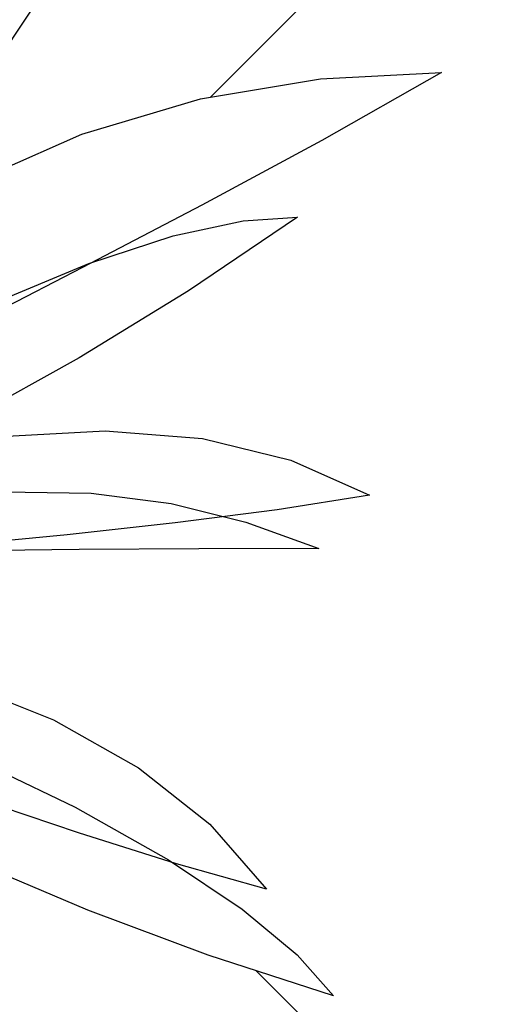
# Model space of a CAD drawing. Units: inches. Extents: x 3590 to 5167, y 65 to 1917.
# Tile 52 of 100: x 4960.64 to 4967.82, y 1515.58 to 1530.53. Entities that reach past the tile are written whole.
import ezdxf

# ---------------------------------------------------------------- set-up
doc = ezdxf.new("R2010")
doc.units = ezdxf.units.IN
doc.layers.add('A-FLOR-PATT', color=8, linetype='Continuous', lineweight=13)
doc.layers.add('L-PLNT', color=94, linetype='Continuous', lineweight=18)
doc.layers.add('DIENHOA', color=3, linetype='Continuous')

# ---------------------------------------------------------------- blocks, each defined once
blk = doc.blocks.new('Cay03_mb')
at = {"layer": 'DIENHOA'}
for p, q in [((510.97, 309.61), (585.91, 313.53)), ((585.91, 313.53), (511.78, 271.41)), ((436.81, 297.21), (510.97, 309.61)), ((363.38, 275.41), (436.81, 297.21)), ((290.63, 243.24), (363.38, 275.41)), ((511.78, 271.41), (437.63, 231.46)), ((437.63, 231.46), (363.69, 192.89)), ((363.69, 192.89), (290.19, 154.87)), ((314.63, 54.14), (369.18, 53.28)), ((369.18, 53.28), (418.6, 46.82)), ((418.6, 46.82), (464.87, 35.24)), ((464.87, 35.24), (510, 19)), ((361.61, 18.5), (289.03, 17.44)), ((435.8, 18.92), (361.61, 18.5)), ((510, 19), (435.8, 18.92)), ((289.55, -107.64), (359.29, -141.1)), ((359.29, -141.1), (416.89, -173.51)), ((367.1, -204.83), (296, -174.69)), ((416.89, -173.51), (462.55, -204.2)), ((441.55, -232.67), (367.1, -204.83)), ((462.55, -204.2), (496.5, -232.48)), ((518.93, -257.68), (441.55, -232.67)), ((496.5, -232.48), (518.93, -257.68))]:
    blk.add_line(p, q, dxfattribs=at)
for points in [[(384.28, 437.45), (342.25, 367.83), (298.14, 301.71), (252.56, 239.37), (206.11, 181.11), (159.39, 127.21), (113.01, 77.96), (67.57, 33.64), (23.69, -5.44)], [(496.74, 224.01), (429.38, 178.44), (361.6, 136.93), (294.07, 99.46), (227.46, 66.07), (162.44, 36.74), (99.68, 11.49), (39.84, -9.67), (-16.39, -26.73)], [(-16.39, -26.73), (75.38, 37.88), (160.06, 91.82), (237.27, 135.67), (306.57, 170.01), (367.58, 195.44), (419.88, 212.52), (463.07, 221.85), (496.74, 224.01)], [(23.69, -5.44), (99.27, 29.67), (173.22, 57.09), (244.79, 76.69), (313.26, 88.31), (377.88, 91.81), (437.93, 87.02), (492.67, 73.8), (541.37, 52)], [(541.37, 52), (484.11, 42.89), (421.18, 34.83), (354.36, 27.58), (285.41, 20.89), (216.1, 14.49), (148.2, 8.14), (83.47, 1.58), (23.69, -5.44)], [(-16.39, -26.73), (66.95, -26.58), (145.58, -32.71), (218.77, -44.94), (285.79, -63.12), (345.92, -87.06), (398.42, -116.6), (442.57, -151.57), (477.63, -191.79)], [(477.63, -191.79), (421.82, -176.03), (361.32, -156.94), (297.62, -135.49), (232.22, -112.64), (166.63, -89.37), (102.33, -66.65), (40.82, -45.45), (-16.39, -26.73)]]:
    blk.add_lwpolyline(points, dxfattribs=at)

msp = doc.modelspace()

# ---------------------------------------------------------------- hatches: boundary and pattern name
at = {"layer": 'A-FLOR-PATT', "transparency": 33554687}
h = msp.add_hatch(dxfattribs=at)
h.set_pattern_fill('AR-HBONE', color=256, scale=0.2)
h.set_pattern_definition([(45, (-588.972, 0), (0, 28.73682), [60.96, -20.32]), (135, (-574.604, 14.368), (3e-15, 28.73682), [60.96, -20.32])])
h.paths.add_polyline_path([(5071.274, 1796.999), (4933.274, 1796.999), (4933.274, 1753.999), (4962.774, 1753.999, -0.414214), (4928.774, 1719.999), (4933.274, 1718.999), (4933.274, 1334.999), (5071.274, 1334.999)])
h.paths.add_polyline_path([(4951.78, 1521.077), (4951.715, 1521.04), (4951.563, 1520.895)], flags=16)
h.paths.add_polyline_path([(4952.267, 1521.376), (4952.198, 1521.371), (4952.198, 1521.356)], flags=0)
h.paths.add_polyline_path([(4967.051, 1529.728), (4965.231, 1528.694), (4963.411, 1527.714), (4961.756, 1526.851), (4963.589, 1527.449), (4964.036, 1527.478), (4962.975, 1527.249), (4961.76, 1526.852), (4959.792, 1525.834), (4958.005, 1524.895), (4956.24, 1523.93), (4954.504, 1522.919), (4954.129, 1522.682), (4953.361, 1521.997), (4953.366, 1521.998), (4953.605, 1522.064), (4955.106, 1522.761), (4956.921, 1523.434), (4958.678, 1523.915), (4960.358, 1524.2), (4961.945, 1524.286), (4964.171, 1524.108), (4965.958, 1523.309), (4963.863, 1522.976), (4965.187, 1522.499), (4963.366, 1522.497), (4961.545, 1522.487), (4959.764, 1522.461), (4958.304, 1522.419), (4957.974, 1522.388), (4956.307, 1522.232), (4954.718, 1522.071), (4953.251, 1521.899), (4953.525, 1521.623), (4954.331, 1521.379), (4956.243, 1521.23), (4958.039, 1520.93), (4959.684, 1520.483), (4961.16, 1519.896), (4963.107, 1518.8), (4964.393, 1517.325), (4962.973, 1517.726), (4964.558, 1516.661), (4965.407, 1515.708), (4963.507, 1516.322), (4961.68, 1517.005), (4959.935, 1517.745), (4958.282, 1518.528), (4956.732, 1519.343), (4955.295, 1520.175), (4954.672, 1520.572), (4954.513, 1520.627), (4955.658, 1519.318), (4956.703, 1517.982), (4957.644, 1516.647), (4958.485, 1515.334), (4959.55, 1513.524), (4960.438, 1511.769), (4958.841, 1513.62), (4957.452, 1515.325), (4955.819, 1517.459), (4956.665, 1515.448), (4957.111, 1513.923), (4957.447, 1511.714), (4957.076, 1509.793), (4956.538, 1511.11), (4955.992, 1512.569), (4955.444, 1514.125), (4954.898, 1515.735), (4954.357, 1517.356), (4953.824, 1518.943), (4953.305, 1520.452), (4953.065, 1521.116), (4952.971, 1521.146), (4952.949, 1521.086), (4952.73, 1520.199), (4953.37, 1518.024), (4953.757, 1516.373), (4954.051, 1514.765), (4954.264, 1513.221), (4954.471, 1511.131), (4954.497, 1510.402), (4954.409, 1511.76), (4954.264, 1513.221), (4954.051, 1514.765), (4953.757, 1516.373), (4953.37, 1518.024), (4952.877, 1519.698), (4952.716, 1520.141), (4952.533, 1519.059), (4952.374, 1517.789), (4952.219, 1516.312), (4952.046, 1514.6), (4951.833, 1512.626), (4951.557, 1510.363), (4951.203, 1512.168), (4950.852, 1514.339), (4950.985, 1516.376), (4951.66, 1518.286), (4952.593, 1520.481), (4952.357, 1521.13), (4951.855, 1520.328), (4950.839, 1518.908), (4949.777, 1517.587), (4948.916, 1516.617), (4948.111, 1515.256), (4947.089, 1513.554), (4945.889, 1511.615), (4946.326, 1513.402), (4946.562, 1514.249), (4945.528, 1513.327), (4944.581, 1512.531), (4946.018, 1514.508), (4947.204, 1516.048), (4947.893, 1517.313), (4949.307, 1518.764), (4950.414, 1519.767), (4950.451, 1519.806), (4952.267, 1521.376), (4951.645, 1521.493), (4950.404, 1521.18), (4948.044, 1520.359), (4946.119, 1519.452), (4944.572, 1518.475), (4943.35, 1517.443), (4941.997, 1515.92), (4941.661, 1515.275), (4942.813, 1516.99), (4944.572, 1518.475), (4946.119, 1519.452), (4948.044, 1520.359), (4950.404, 1521.18), (4951.645, 1521.493), (4949.647, 1521.868), (4948.6, 1521.756), (4947.126, 1521.57), (4945.42, 1521.348), (4943.45, 1521.105), (4941.183, 1520.856), (4942.86, 1521.613), (4943.873, 1522.03), (4942.952, 1521.909), (4941.41, 1521.485), (4939.543, 1520.67), (4938.968, 1520.226), (4940.733, 1521.299), (4942.952, 1521.909), (4943.702, 1522.008), (4945.894, 1522.7), (4947.565, 1522.714), (4948.921, 1522.566), (4951.131, 1522.183), (4950.971, 1522.297), (4948.129, 1523.006), (4946.035, 1523.707), (4944.232, 1524.521), (4942.707, 1525.461), (4941.444, 1526.537), (4940.43, 1527.761), (4939.649, 1529.143), (4941.421, 1528.122), (4943.147, 1527.132), (4944.841, 1526.175), (4946.514, 1525.25), (4948.179, 1524.359), (4948.365, 1524.263), (4946.475, 1526.045), (4945.181, 1527.54), (4944.19, 1529.033), (4943.496, 1530.54), (4943.278, 1531.36), (4942.498, 1531.919), (4943.114, 1531.762), (4942.959, 1533.659), (4944.14, 1531.989), (4944.612, 1531.323), (4946.202, 1530.463), (4947.486, 1529.509), (4948.79, 1528.226), (4950.368, 1526.237), (4949.485, 1528.155), (4948.851, 1530.123), (4948.491, 1532.041), (4948.381, 1533.918), (4948.501, 1535.76), (4948.827, 1537.573), (4949.418, 1535.565), (4949.957, 1533.569), (4950.464, 1531.586), (4950.961, 1529.617), (4951.391, 1527.954), (4951.724, 1530.687), (4952.201, 1532.58), (4952.889, 1534.33), (4953.77, 1535.951), (4954.827, 1537.46), (4954.521, 1535.39), (4954.273, 1533.937), (4955.58, 1535.663), (4956.748, 1536.739), (4956.159, 1534.78), (4955.589, 1532.873), (4955.043, 1531.006), (4954.525, 1529.166), (4954.038, 1527.341), (4953.638, 1525.733), (4953.611, 1525.586), (4953.398, 1524.166), (4953.382, 1524.009), (4954.07, 1525.476), (4954.912, 1527.022), (4956.136, 1528.894), (4957.847, 1530.577), (4959.376, 1531.54), (4958.256, 1530.104), (4957.143, 1528.663), (4956.066, 1527.243), (4955.056, 1525.871), (4954.141, 1524.571), (4953.352, 1523.372), (4953.311, 1523.303), (4953.273, 1522.925), (4953.261, 1522.382), (4954.103, 1523.373), (4954.63, 1524.284), (4955.961, 1526.358), (4957.23, 1528.13), (4958.421, 1529.609), (4960.037, 1531.368), (4961.374, 1532.375), (4962.101, 1532.77), (4961.07, 1531.061), (4959.987, 1529.438), (4958.869, 1527.908), (4958.15, 1527.007), (4959.803, 1528.003), (4961.589, 1528.793), (4963.391, 1529.328), (4965.211, 1529.632)], flags=16)
h.paths.add_polyline_path([(4962.944, 1523.182), (4961.107, 1523.422), (4960.392, 1523.362), (4962.35, 1523.331)], flags=0)
h.paths.add_polyline_path([(5049.541, 1584.551), (5049.476, 1584.515), (5049.325, 1584.37)], flags=16)
h.paths.add_polyline_path([(5050.028, 1584.851), (5049.959, 1584.845), (5049.959, 1584.83)], flags=0)
h.paths.add_polyline_path([(5042.333, 1581.949), (5043.88, 1582.926), (5045.806, 1583.833), (5048.165, 1584.654), (5049.406, 1584.967), (5047.408, 1585.342), (5046.361, 1585.231), (5044.888, 1585.044), (5043.181, 1584.822), (5041.211, 1584.579), (5038.944, 1584.33), (5040.622, 1585.087), (5041.634, 1585.504), (5040.713, 1585.383), (5039.171, 1584.959), (5037.304, 1584.144), (5036.729, 1583.7), (5038.494, 1584.773), (5040.713, 1585.383), (5041.463, 1585.482), (5043.655, 1586.174), (5045.326, 1586.188), (5046.682, 1586.04), (5048.893, 1585.657), (5048.732, 1585.771), (5045.891, 1586.48), (5043.796, 1587.181), (5041.994, 1587.996), (5040.468, 1588.935), (5039.205, 1590.011), (5038.191, 1591.235), (5037.41, 1592.617), (5039.182, 1591.596), (5040.909, 1590.607), (5042.602, 1589.649), (5044.275, 1588.724), (5045.94, 1587.833), (5046.126, 1587.738), (5044.237, 1589.519), (5042.942, 1591.015), (5041.952, 1592.508), (5041.257, 1594.014), (5041.039, 1594.834), (5040.26, 1595.393), (5040.875, 1595.237), (5040.721, 1597.133), (5041.901, 1595.463), (5042.373, 1594.798), (5043.963, 1593.938), (5045.247, 1592.983), (5046.552, 1591.701), (5048.129, 1589.712), (5047.247, 1591.63), (5046.613, 1593.597), (5046.252, 1595.515), (5046.142, 1597.392), (5046.262, 1599.234), (5046.588, 1601.047), (5047.179, 1599.039), (5047.718, 1597.043), (5048.225, 1595.06), (5048.722, 1593.091), (5049.152, 1591.429), (5049.485, 1594.161), (5049.962, 1596.054), (5050.65, 1597.804), (5051.532, 1599.425), (5052.589, 1600.934), (5052.283, 1598.864), (5052.034, 1597.411), (5053.341, 1599.137), (5054.509, 1600.213), (5053.92, 1598.254), (5053.35, 1596.348), (5052.805, 1594.48), (5052.286, 1592.64), (5051.799, 1590.815), (5051.4, 1589.207), (5051.373, 1589.06), (5051.159, 1587.64), (5051.143, 1587.483), (5051.831, 1588.95), (5052.673, 1590.496), (5053.898, 1592.368), (5055.608, 1594.051), (5057.137, 1595.014), (5056.017, 1593.578), (5054.904, 1592.137), (5053.828, 1590.717), (5052.817, 1589.345), (5051.902, 1588.046), (5051.113, 1586.846), (5051.072, 1586.777), (5051.034, 1586.399), (5051.022, 1585.856), (5051.864, 1586.847), (5052.391, 1587.758), (5053.723, 1589.832), (5054.991, 1591.604), (5056.182, 1593.083), (5057.798, 1594.842), (5059.135, 1595.849), (5059.863, 1596.244), (5058.831, 1594.535), (5057.749, 1592.912), (5056.63, 1591.382), (5055.912, 1590.482), (5057.564, 1591.477), (5059.35, 1592.267), (5061.152, 1592.802), (5062.972, 1593.106), (5064.812, 1593.203), (5062.992, 1592.169), (5061.172, 1591.188), (5059.518, 1590.325), (5061.35, 1590.924), (5061.797, 1590.952), (5060.737, 1590.723), (5059.521, 1590.326), (5057.553, 1589.308), (5055.766, 1588.369), (5054.002, 1587.404), (5052.265, 1586.393), (5051.891, 1586.156), (5051.122, 1585.471), (5051.127, 1585.472), (5051.366, 1585.538), (5052.867, 1586.235), (5054.682, 1586.908), (5056.439, 1587.389), (5058.12, 1587.675), (5059.706, 1587.76), (5061.933, 1587.583), (5063.719, 1586.783), (5061.624, 1586.45), (5062.949, 1585.973), (5061.127, 1585.971), (5059.307, 1585.961), (5057.525, 1585.935), (5056.065, 1585.893), (5055.735, 1585.862), (5054.068, 1585.707), (5052.479, 1585.546), (5051.012, 1585.373), (5051.286, 1585.097), (5052.092, 1584.853), (5054.004, 1584.704), (5055.8, 1584.404), (5057.446, 1583.958), (5058.921, 1583.37), (5060.868, 1582.274), (5062.154, 1580.799), (5060.734, 1581.2), (5062.32, 1580.135), (5063.168, 1579.182), (5061.269, 1579.796), (5059.441, 1580.479), (5057.696, 1581.219), (5056.043, 1582.003), (5054.493, 1582.817), (5053.057, 1583.649), (5052.433, 1584.047), (5052.274, 1584.101), (5053.42, 1582.793), (5054.464, 1581.457), (5055.405, 1580.121), (5056.247, 1578.809), (5057.311, 1576.998), (5058.199, 1575.244), (5056.602, 1577.094), (5055.213, 1578.799), (5053.58, 1580.933), (5054.427, 1578.922), (5054.872, 1577.397), (5055.208, 1575.189), (5054.838, 1573.267), (5054.299, 1574.584), (5053.754, 1576.043), (5053.206, 1577.599), (5052.659, 1579.209), (5052.118, 1580.83), (5051.585, 1582.417), (5051.066, 1583.927), (5050.826, 1584.59), (5050.733, 1584.62), (5050.711, 1584.561), (5050.491, 1583.673), (5051.131, 1581.498), (5051.518, 1579.847), (5051.813, 1578.24), (5052.026, 1576.695), (5052.233, 1574.605), (5052.258, 1573.876), (5052.17, 1575.234), (5052.026, 1576.695), (5051.813, 1578.24), (5051.518, 1579.847), (5051.131, 1581.498), (5050.638, 1583.172), (5050.477, 1583.615), (5050.294, 1582.533), (5050.136, 1581.263), (5049.981, 1579.786), (5049.807, 1578.074), (5049.594, 1576.1), (5049.318, 1573.837), (5048.965, 1575.642), (5048.613, 1577.813), (5048.747, 1579.85), (5049.421, 1581.76), (5050.354, 1583.955), (5050.118, 1584.604), (5049.616, 1583.802), (5048.6, 1582.382), (5047.538, 1581.061), (5046.677, 1580.091), (5045.872, 1578.73), (5044.85, 1577.028), (5043.651, 1575.089), (5044.087, 1576.877), (5044.324, 1577.723), (5043.289, 1576.801), (5042.342, 1576.005), (5043.779, 1577.982), (5044.966, 1579.522), (5045.655, 1580.787), (5047.068, 1582.239), (5048.175, 1583.241), (5048.213, 1583.28), (5050.028, 1584.851), (5049.406, 1584.967), (5048.165, 1584.654), (5045.806, 1583.833), (5043.88, 1582.926), (5042.333, 1581.949), (5041.111, 1580.917), (5039.758, 1579.394), (5039.423, 1578.749), (5040.575, 1580.464)], flags=16)
h.paths.add_polyline_path([(4954.799, 1533.12), (4954.262, 1532.079), (4953.831, 1530.935), (4953.505, 1529.636), (4953.283, 1528.133), (4953.167, 1526.376), (4953.156, 1524.315), (4953.277, 1521.236), (4952.802, 1521.842), (4951.557, 1521.998), (4950.976, 1521.961), (4952.661, 1521.941), (4952.802, 1521.842), (4953.152, 1523.593), (4953.167, 1526.376), (4953.283, 1528.133), (4953.609, 1530.346), (4954.456, 1532.592)], flags=0)
h.paths.add_polyline_path([(5050.563, 1585.316), (5049.318, 1585.472), (5048.737, 1585.435), (5050.422, 1585.415), (5050.563, 1585.316), (5050.914, 1587.067), (5050.928, 1589.851), (5051.045, 1591.607), (5051.371, 1593.82), (5052.217, 1596.066), (5052.56, 1596.594), (5052.024, 1595.554), (5051.592, 1594.409), (5051.266, 1593.11), (5051.045, 1591.607), (5050.928, 1589.851), (5050.918, 1587.789), (5051.038, 1584.71)], flags=0)
h.paths.add_polyline_path([(5058.153, 1586.836), (5060.111, 1586.805), (5060.705, 1586.656), (5058.868, 1586.896)], flags=0)
h.paths.add_polyline_path([(5049.541, 1430.936), (5049.476, 1430.9), (5049.325, 1430.755)], flags=16)
h.paths.add_polyline_path([(5050.028, 1431.236), (5049.959, 1431.231), (5049.959, 1431.215)], flags=0)
h.paths.add_polyline_path([(5046.588, 1447.432), (5047.179, 1445.425), (5047.718, 1443.429), (5048.225, 1441.446), (5048.722, 1439.476), (5049.152, 1437.814), (5049.485, 1440.546), (5049.962, 1442.439), (5050.65, 1444.189), (5051.532, 1445.811), (5052.589, 1447.319), (5052.283, 1445.249), (5052.034, 1443.796), (5053.341, 1445.522), (5054.509, 1446.598), (5053.92, 1444.64), (5053.35, 1442.733), (5052.805, 1440.865), (5052.286, 1439.025), (5051.799, 1437.201), (5051.4, 1435.592), (5051.373, 1435.445), (5051.159, 1434.025), (5051.143, 1433.868), (5051.831, 1435.335), (5052.673, 1436.881), (5053.898, 1438.753), (5055.608, 1440.436), (5057.137, 1441.4), (5056.017, 1439.963), (5054.904, 1438.522), (5053.828, 1437.102), (5052.817, 1435.73), (5051.902, 1434.431), (5051.113, 1433.231), (5051.072, 1433.162), (5051.034, 1432.784), (5051.022, 1432.242), (5051.864, 1433.232), (5052.391, 1434.143), (5053.723, 1436.217), (5054.991, 1437.989), (5056.182, 1439.468), (5057.798, 1441.227), (5059.135, 1442.235), (5059.863, 1442.629), (5058.831, 1440.921), (5057.749, 1439.298), (5056.63, 1437.767), (5055.912, 1436.867), (5057.564, 1437.863), (5059.35, 1438.652), (5061.152, 1439.187), (5062.972, 1439.491), (5064.812, 1439.588), (5062.992, 1438.554), (5061.172, 1437.573), (5059.518, 1436.71), (5061.35, 1437.309), (5061.797, 1437.337), (5060.737, 1437.108), (5059.521, 1436.711), (5057.553, 1435.693), (5055.766, 1434.754), (5054.002, 1433.789), (5052.265, 1432.778), (5051.891, 1432.541), (5051.122, 1431.856), (5051.127, 1431.857), (5051.366, 1431.923), (5052.867, 1432.62), (5054.682, 1433.293), (5056.439, 1433.775), (5058.12, 1434.06), (5059.706, 1434.145), (5061.933, 1433.968), (5063.719, 1433.168), (5061.624, 1432.835), (5062.949, 1432.358), (5061.127, 1432.357), (5059.307, 1432.346), (5057.525, 1432.32), (5056.065, 1432.278), (5055.735, 1432.248), (5054.068, 1432.092), (5052.479, 1431.931), (5051.012, 1431.759), (5051.286, 1431.482), (5052.092, 1431.238), (5054.004, 1431.089), (5055.8, 1430.789), (5057.446, 1430.343), (5058.921, 1429.755), (5060.868, 1428.66), (5062.154, 1427.185), (5060.734, 1427.585), (5062.32, 1426.52), (5063.168, 1425.567), (5061.269, 1426.181), (5059.441, 1426.865), (5057.696, 1427.604), (5056.043, 1428.388), (5054.493, 1429.202), (5053.057, 1430.034), (5052.433, 1430.432), (5052.274, 1430.487), (5053.42, 1429.178), (5054.464, 1427.842), (5055.405, 1426.506), (5056.247, 1425.194), (5057.311, 1423.383), (5058.199, 1421.629), (5056.602, 1423.479), (5055.213, 1425.184), (5053.58, 1427.318), (5054.427, 1425.307), (5054.872, 1423.782), (5055.208, 1421.574), (5054.838, 1419.652), (5054.299, 1420.97), (5053.754, 1422.428), (5053.206, 1423.984), (5052.659, 1425.595), (5052.118, 1427.215), (5051.585, 1428.802), (5051.066, 1430.312), (5050.826, 1430.975), (5050.733, 1431.005), (5050.711, 1430.946), (5050.491, 1430.058), (5051.131, 1427.883), (5051.518, 1426.232), (5051.813, 1424.625), (5052.026, 1423.081), (5052.233, 1420.991), (5052.258, 1420.261), (5052.17, 1421.619), (5052.026, 1423.081), (5051.813, 1424.625), (5051.518, 1426.232), (5051.131, 1427.883), (5050.638, 1429.558), (5050.477, 1430.001), (5050.294, 1428.918), (5050.136, 1427.648), (5049.981, 1426.171), (5049.807, 1424.459), (5049.594, 1422.485), (5049.318, 1420.222), (5048.965, 1422.028), (5048.613, 1424.199), (5048.747, 1426.235), (5049.421, 1428.146), (5050.354, 1430.34), (5050.118, 1430.989), (5049.616, 1430.187), (5048.6, 1428.768), (5047.538, 1427.446), (5046.677, 1426.477), (5045.872, 1425.116), (5044.85, 1423.413), (5043.651, 1421.474), (5044.087, 1423.262), (5044.324, 1424.109), (5043.289, 1423.186), (5042.342, 1422.391), (5043.779, 1424.368), (5044.966, 1425.907), (5045.655, 1427.173), (5047.068, 1428.624), (5048.175, 1429.627), (5048.213, 1429.666), (5050.028, 1431.236), (5049.406, 1431.353), (5048.165, 1431.039), (5045.806, 1430.218), (5043.88, 1429.311), (5042.333, 1428.334), (5041.111, 1427.302), (5039.758, 1425.779), (5039.423, 1425.134), (5040.575, 1426.849), (5042.333, 1428.334), (5043.88, 1429.311), (5045.806, 1430.218), (5048.165, 1431.039), (5049.406, 1431.353), (5047.408, 1431.727), (5046.361, 1431.616), (5044.888, 1431.429), (5043.181, 1431.207), (5041.211, 1430.964), (5038.944, 1430.715), (5040.622, 1431.472), (5041.634, 1431.89), (5040.713, 1431.769), (5039.171, 1431.345), (5037.304, 1430.53), (5036.729, 1430.085), (5038.494, 1431.158), (5040.713, 1431.769), (5041.463, 1431.867), (5043.655, 1432.559), (5045.326, 1432.573), (5046.682, 1432.425), (5048.893, 1432.042), (5048.732, 1432.156), (5045.891, 1432.865), (5043.796, 1433.566), (5041.994, 1434.381), (5040.468, 1435.321), (5039.205, 1436.396), (5038.191, 1437.62), (5037.41, 1439.002), (5039.182, 1437.982), (5040.909, 1436.992), (5042.602, 1436.034), (5044.275, 1435.109), (5045.94, 1434.218), (5046.126, 1434.123), (5044.237, 1435.904), (5042.942, 1437.4), (5041.952, 1438.893), (5041.257, 1440.399), (5041.039, 1441.219), (5040.26, 1441.778), (5040.875, 1441.622), (5040.721, 1443.518), (5041.901, 1441.848), (5042.373, 1441.183), (5043.963, 1440.323), (5045.247, 1439.369), (5046.552, 1438.086), (5048.129, 1436.097), (5047.247, 1438.015), (5046.613, 1439.982), (5046.252, 1441.901), (5046.142, 1443.778), (5046.262, 1445.619)], flags=16)
h.paths.add_polyline_path([(5052.382, 1444.255), (5051.623, 1442.78), (5052.024, 1441.939), (5052.56, 1442.98)], flags=0)
h.paths.add_polyline_path([(5050.563, 1431.701), (5049.318, 1431.857), (5048.737, 1431.821), (5050.422, 1431.8)], flags=0)
h.paths.add_polyline_path([(5058.153, 1433.221), (5060.111, 1433.19), (5060.705, 1433.041), (5058.868, 1433.281)], flags=0)
h.paths.add_polyline_path([(5049.541, 1352.285), (5049.476, 1352.249), (5049.325, 1352.104)], flags=16)
h.paths.add_polyline_path([(5050.028, 1352.585), (5049.959, 1352.58), (5049.959, 1352.564)], flags=0)
h.paths.add_polyline_path([(5046.588, 1368.781), (5047.179, 1366.774), (5047.718, 1364.778), (5048.225, 1362.795), (5048.722, 1360.825), (5049.152, 1359.163), (5049.485, 1361.896), (5049.962, 1363.789), (5050.65, 1365.538), (5051.532, 1367.16), (5052.589, 1368.669), (5052.283, 1366.598), (5052.034, 1365.145), (5053.341, 1366.871), (5054.509, 1367.947), (5053.92, 1365.989), (5053.35, 1364.082), (5052.805, 1362.214), (5052.286, 1360.374), (5051.799, 1358.55), (5051.4, 1356.942), (5051.373, 1356.794), (5051.159, 1355.374), (5051.143, 1355.218), (5051.831, 1356.684), (5052.673, 1358.23), (5053.898, 1360.102), (5055.608, 1361.786), (5057.137, 1362.749), (5056.017, 1361.313), (5054.904, 1359.872), (5053.828, 1358.452), (5052.817, 1357.079), (5051.902, 1355.78), (5051.113, 1354.581), (5051.072, 1354.512), (5051.034, 1354.133), (5051.022, 1353.591), (5051.864, 1354.581), (5052.391, 1355.492), (5053.723, 1357.566), (5054.991, 1359.338), (5056.182, 1360.817), (5057.798, 1362.577), (5059.135, 1363.584), (5059.863, 1363.979), (5058.831, 1362.27), (5057.749, 1360.647), (5056.63, 1359.117), (5055.912, 1358.216), (5057.564, 1359.212), (5059.35, 1360.001), (5061.152, 1360.536), (5062.972, 1360.841), (5064.812, 1360.937), (5062.992, 1359.903), (5061.172, 1358.923), (5059.518, 1358.059), (5061.35, 1358.658), (5061.797, 1358.687), (5060.737, 1358.458), (5059.521, 1358.061), (5057.553, 1357.043), (5055.766, 1356.103), (5054.002, 1355.138), (5052.265, 1354.127), (5051.891, 1353.89), (5051.122, 1353.206), (5051.127, 1353.206), (5051.366, 1353.272), (5052.867, 1353.969), (5054.682, 1354.643), (5056.439, 1355.124), (5058.12, 1355.409), (5059.706, 1355.495), (5061.933, 1355.317), (5063.719, 1354.518), (5061.624, 1354.184), (5062.949, 1353.708), (5061.127, 1353.706), (5059.307, 1353.695), (5057.525, 1353.669), (5056.065, 1353.627), (5055.735, 1353.597), (5054.068, 1353.441), (5052.479, 1353.28), (5051.012, 1353.108), (5051.286, 1352.831), (5052.092, 1352.587), (5054.004, 1352.439), (5055.8, 1352.138), (5057.446, 1351.692), (5058.921, 1351.104), (5060.868, 1350.009), (5062.154, 1348.534), (5060.734, 1348.935), (5062.32, 1347.869), (5063.168, 1346.916), (5061.269, 1347.53), (5059.441, 1348.214), (5057.696, 1348.954), (5056.043, 1349.737), (5054.493, 1350.551), (5053.057, 1351.383), (5052.433, 1351.781), (5052.274, 1351.836), (5053.42, 1350.527), (5054.464, 1349.191), (5055.405, 1347.855), (5056.247, 1346.543), (5057.311, 1344.733), (5058.199, 1342.978), (5056.602, 1344.828), (5055.213, 1346.534), (5053.58, 1348.667), (5054.427, 1346.656), (5054.872, 1345.132), (5055.208, 1342.923), (5054.838, 1341.002), (5054.299, 1342.319), (5053.754, 1343.778), (5053.206, 1345.334), (5052.659, 1346.944), (5052.118, 1348.564), (5051.585, 1350.151), (5051.066, 1351.661), (5050.826, 1352.324), (5050.733, 1352.355), (5050.711, 1352.295), (5050.491, 1351.408), (5051.131, 1349.232), (5051.518, 1347.581), (5051.813, 1345.974), (5052.026, 1344.43), (5052.233, 1342.34), (5052.258, 1341.61), (5052.17, 1342.969), (5052.026, 1344.43), (5051.813, 1345.974), (5051.518, 1347.581), (5051.131, 1349.232), (5050.638, 1350.907), (5050.477, 1351.35), (5050.294, 1350.267), (5050.136, 1348.997), (5049.981, 1347.52), (5049.807, 1345.809), (5049.594, 1343.835), (5049.318, 1341.571), (5048.965, 1343.377), (5048.613, 1345.548), (5048.747, 1347.585), (5049.421, 1349.495), (5050.354, 1351.689), (5050.118, 1352.339), (5049.616, 1351.536), (5048.6, 1350.117), (5047.538, 1348.795), (5046.677, 1347.826), (5045.872, 1346.465), (5044.85, 1344.763), (5043.651, 1342.824), (5044.087, 1344.611), (5044.324, 1345.458), (5043.289, 1344.535), (5042.342, 1343.74), (5043.779, 1345.717), (5044.966, 1347.256), (5045.655, 1348.522), (5047.068, 1349.973), (5048.175, 1350.976), (5048.213, 1351.015), (5050.028, 1352.585), (5049.406, 1352.702), (5048.165, 1352.388), (5045.806, 1351.567), (5043.88, 1350.661), (5042.333, 1349.683), (5041.111, 1348.651), (5039.758, 1347.128), (5039.423, 1346.483), (5040.575, 1348.198), (5042.333, 1349.683), (5043.88, 1350.661), (5045.806, 1351.567), (5048.165, 1352.388), (5049.406, 1352.702), (5047.408, 1353.076), (5046.361, 1352.965), (5044.888, 1352.779), (5043.181, 1352.556), (5041.211, 1352.313), (5038.944, 1352.065), (5040.622, 1352.821), (5041.634, 1353.239), (5040.713, 1353.118), (5039.171, 1352.694), (5037.304, 1351.879), (5036.729, 1351.434), (5038.494, 1352.508), (5040.713, 1353.118), (5041.463, 1353.216), (5043.655, 1353.909), (5045.326, 1353.923), (5046.682, 1353.774), (5048.893, 1353.391), (5048.732, 1353.506), (5045.891, 1354.214), (5043.796, 1354.915), (5041.994, 1355.73), (5040.468, 1356.67), (5039.205, 1357.746), (5038.191, 1358.969), (5037.41, 1360.352), (5039.182, 1359.331), (5040.909, 1358.341), (5042.602, 1357.383), (5044.275, 1356.458), (5045.94, 1355.567), (5046.126, 1355.472), (5044.237, 1357.253), (5042.942, 1358.749), (5041.952, 1360.242), (5041.257, 1361.748), (5041.039, 1362.568), (5040.26, 1363.128), (5040.875, 1362.971), (5040.721, 1364.867), (5041.901, 1363.197), (5042.373, 1362.532), (5043.963, 1361.672), (5045.247, 1360.718), (5046.552, 1359.435), (5048.129, 1357.446), (5047.247, 1359.364), (5046.613, 1361.331), (5046.252, 1363.25), (5046.142, 1365.127), (5046.262, 1366.969)], flags=16)
h.paths.add_polyline_path([(5052.382, 1365.604), (5051.623, 1364.129), (5052.024, 1363.288), (5052.56, 1364.329)], flags=0)
h.paths.add_polyline_path([(4951.78, 1698.041), (4951.715, 1698.005), (4951.563, 1697.859)], flags=16)
h.paths.add_polyline_path([(4952.267, 1698.341), (4952.198, 1698.335), (4952.198, 1698.32)], flags=0)
h.paths.add_polyline_path([(4957.076, 1686.757), (4956.538, 1688.074), (4955.992, 1689.533), (4955.444, 1691.089), (4954.898, 1692.699), (4954.357, 1694.32), (4953.824, 1695.907), (4953.305, 1697.417), (4953.065, 1698.08), (4952.971, 1698.11), (4952.949, 1698.051), (4952.73, 1697.163), (4953.37, 1694.988), (4953.757, 1693.337), (4954.051, 1691.729), (4954.264, 1690.185), (4954.471, 1688.095), (4954.497, 1687.366), (4954.409, 1688.724), (4954.264, 1690.185), (4954.051, 1691.729), (4953.757, 1693.337), (4953.37, 1694.988), (4952.877, 1696.662), (4952.716, 1697.105), (4952.533, 1696.023), (4952.374, 1694.753), (4952.219, 1693.276), (4952.046, 1691.564), (4951.833, 1689.59), (4951.557, 1687.327), (4951.203, 1689.132), (4950.852, 1691.303), (4950.985, 1693.34), (4951.66, 1695.25), (4952.593, 1697.445), (4952.357, 1698.094), (4951.855, 1697.292), (4950.839, 1695.872), (4949.777, 1694.551), (4948.916, 1693.581), (4948.111, 1692.22), (4947.089, 1690.518), (4945.889, 1688.579), (4946.326, 1690.366), (4946.562, 1691.213), (4945.528, 1690.291), (4944.581, 1689.495), (4946.018, 1691.472), (4947.204, 1693.012), (4947.893, 1694.277), (4949.307, 1695.729), (4950.414, 1696.731), (4950.451, 1696.77), (4952.267, 1698.341), (4951.645, 1698.457), (4950.404, 1698.144), (4948.044, 1697.323), (4946.119, 1696.416), (4944.572, 1695.439), (4943.35, 1694.407), (4941.997, 1692.884), (4941.661, 1692.239), (4942.813, 1693.954), (4944.572, 1695.439), (4946.119, 1696.416), (4948.044, 1697.323), (4950.404, 1698.144), (4951.645, 1698.457), (4949.647, 1698.832), (4948.6, 1698.72), (4947.126, 1698.534), (4945.42, 1698.312), (4943.45, 1698.069), (4941.183, 1697.82), (4942.86, 1698.577), (4943.873, 1698.994), (4942.952, 1698.873), (4941.41, 1698.449), (4939.543, 1697.634), (4938.968, 1697.19), (4940.733, 1698.263), (4942.952, 1698.873), (4943.702, 1698.972), (4945.894, 1699.664), (4947.565, 1699.678), (4948.921, 1699.53), (4951.131, 1699.147), (4950.971, 1699.261), (4948.129, 1699.97), (4946.035, 1700.671), (4944.232, 1701.486), (4942.707, 1702.425), (4941.444, 1703.501), (4940.43, 1704.725), (4939.649, 1706.107), (4941.421, 1705.086), (4943.147, 1704.097), (4944.841, 1703.139), (4946.514, 1702.214), (4948.179, 1701.323), (4948.365, 1701.227), (4946.475, 1703.009), (4945.181, 1704.505), (4944.19, 1705.997), (4943.496, 1707.504), (4943.278, 1708.324), (4942.498, 1708.883), (4943.114, 1708.727), (4942.959, 1710.623), (4944.14, 1708.953), (4944.612, 1708.287), (4946.202, 1707.428), (4947.486, 1706.473), (4948.79, 1705.191), (4950.368, 1703.202), (4949.485, 1705.12), (4948.851, 1707.087), (4948.491, 1709.005), (4948.381, 1710.882), (4948.501, 1712.724), (4948.827, 1714.537), (4949.418, 1712.529), (4949.957, 1710.533), (4950.464, 1708.55), (4950.961, 1706.581), (4951.391, 1704.919), (4951.724, 1707.651), (4952.201, 1709.544), (4952.889, 1711.294), (4953.77, 1712.915), (4954.827, 1714.424), (4954.521, 1712.354), (4954.273, 1710.901), (4955.58, 1712.627), (4956.748, 1713.703), (4956.159, 1711.744), (4955.589, 1709.837), (4955.043, 1707.97), (4954.525, 1706.13), (4954.038, 1704.305), (4953.638, 1702.697), (4953.611, 1702.55), (4953.398, 1701.13), (4953.382, 1700.973), (4954.07, 1702.44), (4954.912, 1703.986), (4956.136, 1705.858), (4957.847, 1707.541), (4959.376, 1708.504), (4958.256, 1707.068), (4957.143, 1705.627), (4956.066, 1704.207), (4955.056, 1702.835), (4954.141, 1701.536), (4953.352, 1700.336), (4953.311, 1700.267), (4953.273, 1699.889), (4953.261, 1699.346), (4954.103, 1700.337), (4954.63, 1701.248), (4955.961, 1703.322), (4957.23, 1705.094), (4958.421, 1706.573), (4960.037, 1708.332), (4961.374, 1709.339), (4962.101, 1709.734), (4961.07, 1708.025), (4959.987, 1706.402), (4958.869, 1704.872), (4958.15, 1703.972), (4959.803, 1704.967), (4961.589, 1705.757), (4963.391, 1706.292), (4965.211, 1706.596), (4967.051, 1706.692), (4965.231, 1705.659), (4963.411, 1704.678), (4961.756, 1703.815), (4963.589, 1704.413), (4964.036, 1704.442), (4962.975, 1704.213), (4961.76, 1703.816), (4959.792, 1702.798), (4958.005, 1701.859), (4956.24, 1700.894), (4954.504, 1699.883), (4954.129, 1699.646), (4953.361, 1698.961), (4953.366, 1698.962), (4953.605, 1699.028), (4955.106, 1699.725), (4956.921, 1700.398), (4958.678, 1700.879), (4960.358, 1701.164), (4961.945, 1701.25), (4964.171, 1701.073), (4965.958, 1700.273), (4963.863, 1699.94), (4965.187, 1699.463), (4963.366, 1699.461), (4961.545, 1699.451), (4959.764, 1699.425), (4958.304, 1699.383), (4957.974, 1699.352), (4956.307, 1699.197), (4954.718, 1699.036), (4953.251, 1698.863), (4953.525, 1698.587), (4954.331, 1698.343), (4956.243, 1698.194), (4958.039, 1697.894), (4959.684, 1697.447), (4961.16, 1696.86), (4963.107, 1695.764), (4964.393, 1694.289), (4962.973, 1694.69), (4964.558, 1693.625), (4965.407, 1692.672), (4963.507, 1693.286), (4961.68, 1693.969), (4959.935, 1694.709), (4958.282, 1695.492), (4956.732, 1696.307), (4955.295, 1697.139), (4954.672, 1697.536), (4954.513, 1697.591), (4955.658, 1696.282), (4956.703, 1694.946), (4957.644, 1693.611), (4958.485, 1692.298), (4959.55, 1690.488), (4960.438, 1688.733), (4958.841, 1690.584), (4957.452, 1692.289), (4955.819, 1694.423), (4956.665, 1692.412), (4957.111, 1690.887), (4957.447, 1688.678)], flags=16)
h.paths.add_polyline_path([(5050.563, 1353.05), (5049.318, 1353.207), (5048.737, 1353.17), (5050.422, 1353.15)], flags=0)
h.paths.add_polyline_path([(4951.78, 1351.486), (4951.715, 1351.45), (4951.563, 1351.305)], flags=16)
h.paths.add_polyline_path([(4952.267, 1351.786), (4952.198, 1351.78), (4952.198, 1351.765)], flags=0)
h.paths.add_polyline_path([(4954.827, 1367.869), (4954.521, 1365.799), (4954.273, 1364.346), (4955.58, 1366.072), (4956.748, 1367.148), (4956.159, 1365.19), (4955.589, 1363.283), (4955.043, 1361.415), (4954.525, 1359.575), (4954.038, 1357.751), (4953.638, 1356.142), (4953.611, 1355.995), (4953.398, 1354.575), (4953.382, 1354.418), (4954.07, 1355.885), (4954.912, 1357.431), (4956.136, 1359.303), (4957.847, 1360.986), (4959.376, 1361.95), (4958.256, 1360.513), (4957.143, 1359.072), (4956.066, 1357.652), (4955.056, 1356.28), (4954.141, 1354.981), (4953.352, 1353.781), (4953.311, 1353.712), (4953.273, 1353.334), (4953.261, 1352.792), (4954.103, 1353.782), (4954.63, 1354.693), (4955.961, 1356.767), (4957.23, 1358.539), (4958.421, 1360.018), (4960.037, 1361.777), (4961.374, 1362.785), (4962.101, 1363.179), (4961.07, 1361.471), (4959.987, 1359.848), (4958.869, 1358.317), (4958.15, 1357.417), (4959.803, 1358.413), (4961.589, 1359.202), (4963.391, 1359.737), (4965.211, 1360.041), (4967.051, 1360.138), (4965.231, 1359.104), (4963.411, 1358.123), (4961.756, 1357.26), (4963.589, 1357.859), (4964.036, 1357.887), (4962.975, 1357.658), (4961.76, 1357.261), (4959.792, 1356.243), (4958.005, 1355.304), (4956.24, 1354.339), (4954.504, 1353.328), (4954.129, 1353.091), (4953.361, 1352.406), (4953.366, 1352.407), (4953.605, 1352.473), (4955.106, 1353.17), (4956.921, 1353.843), (4958.678, 1354.325), (4960.358, 1354.61), (4961.945, 1354.695), (4964.171, 1354.518), (4965.958, 1353.718), (4963.863, 1353.385), (4965.187, 1352.908), (4963.366, 1352.907), (4961.545, 1352.896), (4959.764, 1352.87), (4958.304, 1352.828), (4957.974, 1352.798), (4956.307, 1352.642), (4954.718, 1352.481), (4953.251, 1352.309), (4953.525, 1352.032), (4954.331, 1351.788), (4956.243, 1351.639), (4958.039, 1351.339), (4959.684, 1350.893), (4961.16, 1350.305), (4963.107, 1349.21), (4964.393, 1347.735), (4962.973, 1348.135), (4964.558, 1347.07), (4965.407, 1346.117), (4963.507, 1346.731), (4961.68, 1347.414), (4959.935, 1348.154), (4958.282, 1348.938), (4956.732, 1349.752), (4955.295, 1350.584), (4954.672, 1350.982), (4954.513, 1351.036), (4955.658, 1349.728), (4956.703, 1348.392), (4957.644, 1347.056), (4958.485, 1345.744), (4959.55, 1343.933), (4960.438, 1342.179), (4958.841, 1344.029), (4957.452, 1345.734), (4955.819, 1347.868), (4956.665, 1345.857), (4957.111, 1344.332), (4957.447, 1342.124), (4957.076, 1340.202), (4956.538, 1341.52), (4955.992, 1342.978), (4955.444, 1344.534), (4954.898, 1346.145), (4954.357, 1347.765), (4953.824, 1349.352), (4953.305, 1350.862), (4953.065, 1351.525), (4952.971, 1351.555), (4952.949, 1351.496), (4952.73, 1350.608), (4953.37, 1348.433), (4953.757, 1346.782), (4954.051, 1345.175), (4954.264, 1343.631), (4954.471, 1341.541), (4954.497, 1340.811), (4954.409, 1342.169), (4954.264, 1343.631), (4954.051, 1345.175), (4953.757, 1346.782), (4953.37, 1348.433), (4952.877, 1350.108), (4952.716, 1350.551), (4952.533, 1349.468), (4952.374, 1348.198), (4952.219, 1346.721), (4952.046, 1345.009), (4951.833, 1343.035), (4951.557, 1340.772), (4951.203, 1342.578), (4950.852, 1344.749), (4950.985, 1346.785), (4951.66, 1348.696), (4952.593, 1350.89), (4952.357, 1351.539), (4951.855, 1350.737), (4950.839, 1349.318), (4949.777, 1347.996), (4948.916, 1347.027), (4948.111, 1345.665), (4947.089, 1343.963), (4945.889, 1342.024), (4946.326, 1343.812), (4946.562, 1344.659), (4945.528, 1343.736), (4944.581, 1342.941), (4946.018, 1344.918), (4947.204, 1346.457), (4947.893, 1347.723), (4949.307, 1349.174), (4950.414, 1350.177), (4950.451, 1350.216), (4952.267, 1351.786), (4951.645, 1351.903), (4950.404, 1351.589), (4948.044, 1350.768), (4946.119, 1349.861), (4944.572, 1348.884), (4943.35, 1347.852), (4941.997, 1346.329), (4941.661, 1345.684), (4942.813, 1347.399), (4944.572, 1348.884), (4946.119, 1349.861), (4948.044, 1350.768), (4950.404, 1351.589), (4951.645, 1351.903), (4949.647, 1352.277), (4948.6, 1352.166), (4947.126, 1351.979), (4945.42, 1351.757), (4943.45, 1351.514), (4941.183, 1351.265), (4942.86, 1352.022), (4943.873, 1352.44), (4942.952, 1352.319), (4941.41, 1351.895), (4939.543, 1351.08), (4938.968, 1350.635), (4940.733, 1351.708), (4942.952, 1352.319), (4943.702, 1352.417), (4945.894, 1353.109), (4947.565, 1353.123), (4948.921, 1352.975), (4951.131, 1352.592), (4950.971, 1352.706), (4948.129, 1353.415), (4946.035, 1354.116), (4944.232, 1354.931), (4942.707, 1355.871), (4941.444, 1356.946), (4940.43, 1358.17), (4939.649, 1359.552), (4941.421, 1358.532), (4943.147, 1357.542), (4944.841, 1356.584), (4946.514, 1355.659), (4948.179, 1354.768), (4948.365, 1354.673), (4946.475, 1356.454), (4945.181, 1357.95), (4944.19, 1359.443), (4943.496, 1360.949), (4943.278, 1361.769), (4942.498, 1362.328), (4943.114, 1362.172), (4942.959, 1364.068), (4944.14, 1362.398), (4944.612, 1361.733), (4946.202, 1360.873), (4947.486, 1359.919), (4948.79, 1358.636), (4950.368, 1356.647), (4949.485, 1358.565), (4948.851, 1360.532), (4948.491, 1362.451), (4948.381, 1364.328), (4948.501, 1366.169), (4948.827, 1367.982), (4949.418, 1365.975), (4949.957, 1363.979), (4950.464, 1361.995), (4950.961, 1360.026), (4951.391, 1358.364), (4951.724, 1361.096), (4952.201, 1362.989), (4952.889, 1364.739), (4953.77, 1366.361)], flags=16)
h.paths.add_polyline_path([(4954.799, 1363.53), (4954.262, 1362.489), (4953.831, 1361.344), (4953.505, 1360.045), (4953.283, 1358.543), (4953.167, 1356.786), (4953.156, 1354.724), (4953.277, 1351.646), (4952.802, 1352.251), (4951.557, 1352.407), (4950.976, 1352.371), (4952.661, 1352.35), (4952.802, 1352.251), (4953.152, 1354.002), (4953.167, 1356.786), (4953.283, 1358.543), (4953.609, 1360.755), (4954.456, 1363.001)], flags=0)
h.paths.add_polyline_path([(4952.802, 1698.806), (4951.557, 1698.962), (4950.976, 1698.925), (4952.661, 1698.905), (4952.802, 1698.806), (4953.152, 1700.557), (4953.167, 1703.34), (4953.283, 1705.097), (4953.609, 1707.31), (4954.456, 1709.556), (4954.799, 1710.084), (4954.262, 1709.043), (4953.831, 1707.899), (4953.505, 1706.6), (4953.283, 1705.097), (4953.167, 1703.34), (4953.156, 1701.279), (4953.277, 1698.2)], flags=0)
h.paths.add_polyline_path([(4962.944, 1700.146), (4961.107, 1700.386), (4960.392, 1700.326), (4962.35, 1700.295)], flags=0)
h.paths.add_polyline_path([(5058.153, 1354.57), (5060.111, 1354.539), (5060.705, 1354.391), (5058.868, 1354.631)], flags=0)
h.paths.add_polyline_path([(4962.944, 1353.591), (4961.107, 1353.831), (4960.392, 1353.771), (4962.35, 1353.74)], flags=0)
h.paths.add_polyline_path([(5049.541, 1778.72), (5049.476, 1778.684), (5049.325, 1778.539)], flags=16)
h.paths.add_polyline_path([(5050.028, 1779.02), (5049.959, 1779.014), (5049.959, 1778.999)], flags=0)
h.paths.add_polyline_path([(5052.258, 1768.045), (5052.17, 1769.403), (5052.026, 1770.864), (5051.813, 1772.409), (5051.518, 1774.016), (5051.131, 1775.667), (5050.638, 1777.341), (5050.477, 1777.784), (5050.294, 1776.702), (5050.136, 1775.432), (5049.981, 1773.955), (5049.807, 1772.243), (5049.594, 1770.269), (5049.318, 1768.006), (5048.965, 1769.811), (5048.613, 1771.982), (5048.747, 1774.019), (5049.421, 1775.929), (5050.354, 1778.124), (5050.118, 1778.773), (5049.616, 1777.971), (5048.6, 1776.551), (5047.538, 1775.23), (5046.677, 1774.26), (5045.872, 1772.899), (5044.85, 1771.197), (5043.651, 1769.258), (5044.087, 1771.046), (5044.324, 1771.892), (5043.289, 1770.97), (5042.342, 1770.174), (5043.779, 1772.151), (5044.966, 1773.691), (5045.655, 1774.956), (5047.068, 1776.408), (5048.175, 1777.41), (5048.213, 1777.449), (5050.028, 1779.02), (5049.406, 1779.136), (5048.165, 1778.823), (5045.806, 1778.002), (5043.88, 1777.095), (5042.333, 1776.118), (5041.111, 1775.086), (5039.758, 1773.563), (5039.423, 1772.918), (5040.575, 1774.633), (5042.333, 1776.118), (5043.88, 1777.095), (5045.806, 1778.002), (5048.165, 1778.823), (5049.406, 1779.136), (5047.408, 1779.511), (5046.361, 1779.4), (5044.888, 1779.213), (5043.181, 1778.991), (5041.211, 1778.748), (5038.944, 1778.499), (5040.622, 1779.256), (5041.634, 1779.673), (5040.713, 1779.552), (5039.171, 1779.128), (5037.304, 1778.313), (5036.729, 1777.869), (5038.494, 1778.942), (5040.713, 1779.552), (5041.463, 1779.651), (5043.655, 1780.343), (5045.326, 1780.357), (5046.682, 1780.209), (5048.893, 1779.826), (5048.732, 1779.94), (5045.891, 1780.649), (5043.796, 1781.35), (5041.994, 1782.165), (5040.468, 1783.104), (5039.205, 1784.18), (5038.191, 1785.404), (5037.41, 1786.786), (5039.182, 1785.765), (5040.909, 1784.776), (5042.602, 1783.818), (5044.275, 1782.893), (5045.94, 1782.002), (5046.126, 1781.907), (5044.237, 1783.688), (5042.942, 1785.184), (5041.952, 1786.677), (5041.257, 1788.183), (5041.039, 1789.003), (5040.26, 1789.562), (5040.875, 1789.406), (5040.721, 1791.302), (5041.901, 1789.632), (5042.373, 1788.967), (5043.963, 1788.107), (5045.247, 1787.152), (5046.552, 1785.87), (5048.129, 1783.881), (5047.247, 1785.799), (5046.613, 1787.766), (5046.252, 1789.684), (5046.142, 1791.561), (5046.262, 1793.403), (5046.588, 1795.216), (5047.179, 1793.208), (5047.718, 1791.213), (5048.225, 1789.229), (5048.722, 1787.26), (5049.152, 1785.598), (5049.485, 1788.33), (5049.962, 1790.223), (5050.65, 1791.973), (5051.532, 1793.594), (5052.589, 1795.103), (5052.283, 1793.033), (5052.034, 1791.58), (5053.341, 1793.306), (5054.509, 1794.382), (5053.92, 1792.423), (5053.35, 1790.517), (5052.805, 1788.649), (5052.286, 1786.809), (5051.799, 1784.984), (5051.4, 1783.376), (5051.373, 1783.229), (5051.159, 1781.809), (5051.143, 1781.652), (5051.831, 1783.119), (5052.673, 1784.665), (5053.898, 1786.537), (5055.608, 1788.22), (5057.137, 1789.183), (5056.017, 1787.747), (5054.904, 1786.306), (5053.828, 1784.886), (5052.817, 1783.514), (5051.902, 1782.215), (5051.113, 1781.015), (5051.072, 1780.946), (5051.034, 1780.568), (5051.022, 1780.025), (5051.864, 1781.016), (5052.391, 1781.927), (5053.723, 1784.001), (5054.991, 1785.773), (5056.182, 1787.252), (5057.798, 1789.011), (5059.135, 1790.018), (5059.863, 1790.413), (5058.831, 1788.704), (5057.749, 1787.081), (5056.63, 1785.551), (5055.912, 1784.651), (5057.564, 1785.646), (5059.35, 1786.436), (5061.152, 1786.971), (5062.972, 1787.275), (5064.812, 1787.372), (5062.992, 1786.338), (5061.172, 1785.357), (5059.518, 1784.494), (5061.35, 1785.093), (5061.797, 1785.121), (5060.737, 1784.892), (5059.521, 1784.495), (5057.553, 1783.477), (5055.766, 1782.538), (5054.002, 1781.573), (5052.265, 1780.562), (5051.891, 1780.325), (5051.122, 1779.64), (5051.127, 1779.641), (5051.366, 1779.707), (5052.867, 1780.404), (5054.682, 1781.077), (5056.439, 1781.558), (5058.12, 1781.844), (5059.706, 1781.929), (5061.933, 1781.752), (5063.719, 1780.952), (5061.624, 1780.619), (5062.949, 1780.142), (5061.127, 1780.14), (5059.307, 1780.13), (5057.525, 1780.104), (5056.065, 1780.062), (5055.735, 1780.031), (5054.068, 1779.876), (5052.479, 1779.715), (5051.012, 1779.542), (5051.286, 1779.266), (5052.092, 1779.022), (5054.004, 1778.873), (5055.8, 1778.573), (5057.446, 1778.127), (5058.921, 1777.539), (5060.868, 1776.443), (5062.154, 1774.968), (5060.734, 1775.369), (5062.32, 1774.304), (5063.168, 1773.351), (5061.269, 1773.965), (5059.441, 1774.648), (5057.696, 1775.388), (5056.043, 1776.172), (5054.493, 1776.986), (5053.057, 1777.818), (5052.433, 1778.216), (5052.274, 1778.27), (5053.42, 1776.962), (5054.464, 1775.626), (5055.405, 1774.29), (5056.247, 1772.978), (5057.311, 1771.167), (5058.199, 1769.413), (5056.602, 1771.263), (5055.213, 1772.968), (5053.58, 1775.102), (5054.427, 1773.091), (5054.872, 1771.566), (5055.208, 1769.358), (5054.838, 1767.436), (5054.299, 1768.753), (5053.754, 1770.212), (5053.206, 1771.768), (5052.659, 1773.378), (5052.118, 1774.999), (5051.585, 1776.586), (5051.066, 1778.096), (5050.826, 1778.759), (5050.733, 1778.789), (5050.711, 1778.73), (5050.491, 1777.842), (5051.131, 1775.667), (5051.518, 1774.016), (5051.813, 1772.409), (5052.026, 1770.864), (5052.233, 1768.774)], flags=16)
h.paths.add_polyline_path([(5050.563, 1779.485), (5049.318, 1779.641), (5048.737, 1779.604), (5050.422, 1779.584), (5050.563, 1779.485), (5050.914, 1781.236), (5050.928, 1784.02), (5051.045, 1785.776), (5051.371, 1787.989), (5052.217, 1790.235), (5052.56, 1790.763), (5052.024, 1789.723), (5051.592, 1788.578), (5051.266, 1787.279), (5051.045, 1785.776), (5050.928, 1784.02), (5050.918, 1781.958), (5051.038, 1778.879)], flags=0)
h.paths.add_polyline_path([(5058.153, 1781.005), (5060.111, 1780.974), (5060.705, 1780.825), (5058.868, 1781.065)], flags=0)

# ---------------------------------------------------------------- block references
at = {"layer": 'L-PLNT', "xscale": 0.0245452446402784, "yscale": 0.0245452446402784, "zscale": 0.0245452446402784}
msp.add_blockref('Cay03_mb', (4952.669, 1522.033), dxfattribs=at)

doc.saveas('drawing.dxf')
